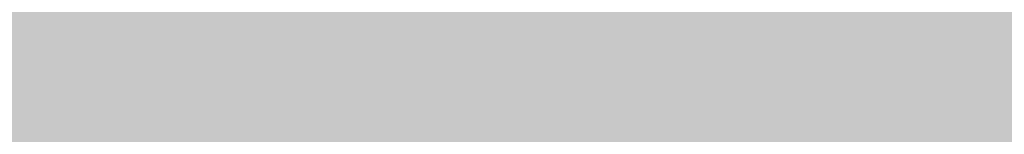
# Model space of a CAD drawing. Units: millimetres. Extents: x 0 to 2267, y 0 to 1823.
# Tile 174 of 256: x 1833.606 to 1838.83, y 1127.888 to 1128.496. Entities that reach past the tile are written whole.
import ezdxf

# ---------------------------------------------------------------- set-up
doc = ezdxf.new("R2010")
doc.units = ezdxf.units.MM
doc.header["$MEASUREMENT"] = 0
doc.layers.add('M-HATC', color=252, linetype='Continuous', lineweight=18)

msp = doc.modelspace()

# ---------------------------------------------------------------- hatches: boundary and pattern name
at = {"layer": 'M-HATC'}
h = msp.add_hatch(color=256, dxfattribs=at)
h.dxf.hatch_style = 1
h.paths.add_polyline_path([(2055.771, 1603.062), (1381.0868, 1603.062), (1381.0868, 1598.062), (2055.771, 1598.062)])
h.paths.add_polyline_path([(2055.771, 1598.062), (1381.0868, 1598.062), (1381.0868, 1593.062), (2055.771, 1593.062)])
h.paths.add_polyline_path([(2051.3074, 1536.7609), (1385.5504, 1536.7609), (1385.5504, 1526.7609), (1387.5504, 1526.7609), (1388.5366, 1525.0528), (1385.3319, 1521.2335), (1385.3319, 1521.2226), (2050.2542, 1522.7491), (2048.3212, 1525.0528), (2049.3074, 1526.7609), (2051.3074, 1526.7609)])
edge = h.paths.add_edge_path()
edge.add_arc((1847.5345, 1379.1492), 135, 222.603061, 222.890851, ccw=False)
edge.add_line((1748.1663, 1287.7656), (1683.0921, 1287.7656))
edge.add_arc((1583.7239, 1379.1492), 135, 317.109149, 317.396939, ccw=False)
edge.add_arc((1678.9686, 1290.6707), 5, 222.8909, 317.1091, ccw=False)
edge.add_arc((1774.2133, 1379.1492), 135, 222.603061, 222.890851, ccw=False)
edge.add_line((1674.8451, 1287.7656), (1609.7709, 1287.7656))
edge.add_arc((1510.4027, 1379.1492), 135, 317.109149, 317.396939, ccw=False)
edge.add_arc((1605.6474, 1290.6707), 5, 222.8909, 317.1091, ccw=False)
edge.add_arc((1700.8921, 1379.1492), 135, 222.603061, 222.890851, ccw=False)
edge.add_line((1601.5239, 1287.7656), (1536.4497, 1287.7656))
edge.add_arc((1437.0815, 1379.1492), 135, 317.109149, 317.396939, ccw=False)
edge.add_arc((1532.3262, 1290.6707), 5, 222.8909, 317.1091, ccw=False)
edge.add_arc((1627.5709, 1379.1492), 135, 222.603061, 222.890851, ccw=False)
edge.add_line((1528.2027, 1287.7656), (1505.9289, 1287.7656))
edge.add_spline(control_points=[(1505.9289, 1287.7656), (1504.2622, 1287.7656), (1504.2622, 1282.7656), (1505.9289, 1282.7656)], knot_values=[0, 0, 0, 0, 5, 5, 5, 5], degree=3, periodic=0)
edge.add_line((1505.9289, 1282.7656), (1930.9289, 1282.7656))
edge.add_spline(control_points=[(1930.9289, 1282.7656), (1932.5956, 1282.7656), (1932.5956, 1287.7656), (1930.9289, 1287.7656)], knot_values=[0, 0, 0, 0, 5, 5, 5, 5], degree=3, periodic=0)
edge.add_line((1930.9289, 1287.7656), (1903.0557, 1287.7656))
edge.add_arc((1803.6875, 1379.1492), 135, 317.109149, 317.396939, ccw=False)
edge.add_arc((1898.9322, 1290.6707), 5, 222.8909, 317.1091, ccw=False)
edge.add_arc((1994.1769, 1379.1492), 135, 222.603061, 222.890851, ccw=False)
edge.add_line((1894.8087, 1287.7656), (1829.7345, 1287.7656))
edge.add_arc((1730.3663, 1379.1492), 135, 317.109149, 317.396939, ccw=False)
edge.add_arc((1825.611, 1290.6707), 5, 222.8909, 317.1091, ccw=False)
edge.add_arc((1920.8557, 1379.1492), 135, 222.603061, 222.890851, ccw=False)
edge.add_line((1821.4875, 1287.7656), (1756.4133, 1287.7656))
edge.add_arc((1657.0451, 1379.1492), 135, 317.109149, 317.396939, ccw=False)
edge.add_arc((1752.2898, 1290.6707), 5, 222.8909, 317.1091, ccw=False)
edge = h.paths.add_edge_path()
edge.add_spline(control_points=[(1843.4289, 1227.2475), (1845.0956, 1227.2475), (1845.0956, 1232.2475), (1843.4289, 1232.2475)], knot_values=[0, 0, 0, 0, 5, 5, 5, 5], degree=3, periodic=0)
edge.add_line((1843.4289, 1232.2475), (1593.4289, 1232.2475))
edge.add_spline(control_points=[(1593.4289, 1232.2475), (1591.7622, 1232.2475), (1591.7622, 1227.2475), (1593.4289, 1227.2475)], knot_values=[0, 0, 0, 0, 5, 5, 5, 5], degree=3, periodic=0)
edge.add_line((1593.4289, 1227.2475), (1843.4289, 1227.2475))
h.paths.add_polyline_path([(1905.9289, 1127.4171), (1530.9289, 1127.4171, 0.414214), (1520.9289, 1117.4171), (1530.9289, 1117.4171), (1915.9289, 1117.4171, 0.414214)])
edge = h.paths.add_edge_path()
edge.add_arc((1397.0858, 1498.4078), 12.7299, 90.78215, 190.87871, ccw=False)
edge.add_line((1396.912, 1511.1365), (1428.0097, 1511.3488))
edge.add_line((1428.0097, 1511.3488), (1433.0097, 1511.3488))
edge.add_line((1433.0097, 1511.3488), (1434.439, 1511.3488))
edge.add_arc((1419.474, 1498.0804), 20, 41.561, 74.08211)
edge.add_line((1424.9592, 1517.3135), (1399.9351, 1517.2561))
edge.add_spline(control_points=[(1399.9307, 1517.2561), (1399.884, 1517.2131), (1399.8328, 1517.1689), (1399.7774, 1517.1236)], knot_values=[11.567499, 11.567499, 11.567499, 11.567499, 11.814249, 11.814249, 11.814249, 11.814249], degree=3, periodic=0)
edge.add_spline(control_points=[(1399.6328, 1517.0099), (1399.5831, 1516.9721), (1399.5307, 1516.9338), (1399.4759, 1516.8947)], knot_values=[11.167718, 11.167718, 11.167718, 11.167718, 11.365188, 11.365188, 11.365188, 11.365188], degree=3, periodic=0)
edge.add_spline(control_points=[(1399.3398, 1516.8001), (1399.1514, 1516.6719), (1398.9384, 1516.5377), (1398.704, 1516.3994)], knot_values=[10.376405, 10.376405, 10.376405, 10.376405, 11.00994, 11.00994, 11.00994, 11.00994], degree=3, periodic=0)
edge.add_spline(control_points=[(1398.6572, 1516.3719), (1398.5789, 1516.326), (1398.4983, 1516.2797), (1398.4155, 1516.2331)], knot_values=[10.125175, 10.125175, 10.125175, 10.125175, 10.334406, 10.334406, 10.334406, 10.334406], degree=3, periodic=0)
edge.add_spline(control_points=[(1398.2642, 1516.1487), (1398.196, 1516.1111), (1398.1263, 1516.0732), (1398.0555, 1516.0351)], knot_values=[9.832246, 9.832246, 9.832246, 9.832246, 9.999658, 9.999658, 9.999658, 9.999658], degree=3, periodic=0)
edge.add_spline(control_points=[(1397.9987, 1516.0048), (1397.7312, 1515.8621), (1397.446, 1515.7171), (1397.1466, 1515.5714)], knot_values=[9.161808, 9.161808, 9.161808, 9.161808, 9.787769, 9.787769, 9.787769, 9.787769], degree=3, periodic=0)
edge.add_spline(control_points=[(1397.1466, 1515.5714), (1396.8418, 1515.423), (1396.5222, 1515.274), (1396.1914, 1515.1262)], knot_values=[8.524455, 8.524455, 8.524455, 8.524455, 9.161808, 9.161808, 9.161808, 9.161808], degree=3, periodic=0)
edge.add_spline(control_points=[(1396.0777, 1515.0756), (1395.9854, 1515.0348), (1395.8922, 1514.994), (1395.7983, 1514.9534)], knot_values=[8.275193, 8.275193, 8.275193, 8.275193, 8.451726, 8.451726, 8.451726, 8.451726], degree=3, periodic=0)
edge.add_spline(control_points=[(1395.6018, 1514.8691), (1395.4997, 1514.8257), (1395.3968, 1514.7824), (1395.2932, 1514.7394)], knot_values=[7.962917, 7.962917, 7.962917, 7.962917, 8.152764, 8.152764, 8.152764, 8.152764], degree=3, periodic=0)
edge.add_spline(control_points=[(1395.2116, 1514.7057), (1394.8278, 1514.5475), (1394.4345, 1514.3929), (1394.0364, 1514.2442)], knot_values=[7.21254, 7.21254, 7.21254, 7.21254, 7.913148, 7.913148, 7.913148, 7.913148], degree=3, periodic=0)
edge.add_spline(control_points=[(1394.0364, 1514.2442), (1393.7076, 1514.1214), (1393.3754, 1514.0027), (1393.0427, 1513.8895)], knot_values=[6.633733, 6.633733, 6.633733, 6.633733, 7.21254, 7.21254, 7.21254, 7.21254], degree=3, periodic=0)
edge.add_spline(control_points=[(1392.8214, 1513.815), (1392.7198, 1513.7812), (1392.6181, 1513.7479), (1392.5166, 1513.7152)], knot_values=[6.328796, 6.328796, 6.328796, 6.328796, 6.505493, 6.505493, 6.505493, 6.505493], degree=3, periodic=0)
edge.add_spline(control_points=[(1392.5166, 1513.7152), (1392.3187, 1513.6515), (1392.1212, 1513.59), (1391.9244, 1513.531)], knot_values=[5.984605, 5.984605, 5.984605, 5.984605, 6.328796, 6.328796, 6.328796, 6.328796], degree=3, periodic=0)
edge.add_spline(control_points=[(1391.7915, 1513.4915), (1391.3122, 1513.3501), (1390.8384, 1513.2239), (1390.3784, 1513.1171)], knot_values=[5.066697, 5.066697, 5.066697, 5.066697, 5.907055, 5.907055, 5.907055, 5.907055], degree=3, periodic=0)
edge.add_spline(control_points=[(1390.3784, 1513.1171), (1390.1797, 1513.071), (1389.9836, 1513.0284), (1389.7907, 1512.9899)], knot_values=[4.70367, 4.70367, 4.70367, 4.70367, 5.066695, 5.066695, 5.066695, 5.066695], degree=3, periodic=0)
edge.add_spline(control_points=[(1389.422, 1512.9204), (1389.2459, 1512.8892), (1389.0729, 1512.8617), (1388.9036, 1512.8381)], knot_values=[4.130571, 4.130571, 4.130571, 4.130571, 4.469816, 4.469816, 4.469816, 4.469816], degree=3, periodic=0)
edge.add_spline(control_points=[(1388.9036, 1512.8381), (1388.591, 1512.7946), (1388.2911, 1512.7644), (1388.0071, 1512.7494)], knot_values=[3.504031, 3.504031, 3.504031, 3.504031, 4.130571, 4.130571, 4.130571, 4.130571], degree=3, periodic=0)
edge.add_spline(control_points=[(1387.9356, 1512.7459), (1387.8538, 1512.7423), (1387.7733, 1512.74), (1387.6944, 1512.739)], knot_values=[3.268866, 3.268866, 3.268866, 3.268866, 3.451164, 3.451164, 3.451164, 3.451164], degree=3, periodic=0)
edge.add_spline(control_points=[(1387.3351, 1512.7443), (1387.2076, 1512.7499), (1387.0847, 1512.7597), (1386.967, 1512.7739)], knot_values=[2.670686, 2.670686, 2.670686, 2.670686, 2.984, 2.984, 2.984, 2.984], degree=3, periodic=0)
edge.add_spline(control_points=[(1386.8327, 1512.7922), (1386.8209, 1512.7941), (1386.8092, 1512.7959), (1386.7975, 1512.7979)], knot_values=[2.516981, 2.516981, 2.516981, 2.516981, 2.549528, 2.549528, 2.549528, 2.549528], degree=3, periodic=0)
edge.add_spline(control_points=[(1386.4526, 1512.8735), (1386.4257, 1512.881), (1386.3993, 1512.889), (1386.3733, 1512.8972)], knot_values=[2.095869, 2.095869, 2.095869, 2.095869, 2.17941, 2.17941, 2.17941, 2.17941], degree=3, periodic=0)
edge.add_spline(control_points=[(1386.0691, 1513.0189), (1386.0634, 1513.0217), (1386.0577, 1513.0246), (1386.052, 1513.0275)], knot_values=[1.72453, 1.72453, 1.72453, 1.72453, 1.745933, 1.745933, 1.745933, 1.745933], degree=3, periodic=0)
edge.add_arc((1399.474, 1498.0804), 20, 131.82432, 180)
edge.add_arc((1630.3336, 1505.5484), 250.9708, 181.705176, 236.427975)
edge.add_arc((1605.3399, 1483.3044), 218.7822, 238.660829, 243.34961)
edge.add_arc((1647.0911, 1510.3592), 262.8986, 183.129836, 237.853442, ccw=False)
h.paths.add_polyline_path([(1406.5369, 1391.9644, 0.149382), (1491.5506, 1296.4418, -0.129517)], flags=17)
edge = h.paths.add_edge_path()
edge.add_arc((2037.3838, 1498.0804), 20, 0, 48.26587)
edge.add_spline(control_points=[(2050.6973, 1513.0052), (2050.6512, 1512.9847), (2050.6034, 1512.9655), (2050.5539, 1512.9477)], knot_values=[1.835652, 1.835652, 1.835652, 1.835652, 2.000781, 2.000781, 2.000781, 2.000781], degree=3, periodic=0)
edge.add_spline(control_points=[(2050.4616, 1512.9166), (2050.479, 1512.9221), (2050.4963, 1512.9277), (2050.5133, 1512.9335)], knot_values=[2.045477, 2.045477, 2.045477, 2.045477, 2.101389, 2.101389, 2.101389, 2.101389], degree=3, periodic=0)
edge.add_spline(control_points=[(2050.129, 1512.8342), (2050.1984, 1512.8473), (2050.2657, 1512.8623), (2050.3308, 1512.8792)], knot_values=[2.237629, 2.237629, 2.237629, 2.237629, 2.435841, 2.435841, 2.435841, 2.435841], degree=3, periodic=0)
edge.add_spline(control_points=[(2050.0946, 1512.8278), (2050.1061, 1512.8299), (2050.1176, 1512.832), (2050.129, 1512.8342)], knot_values=[2.435841, 2.435841, 2.435841, 2.435841, 2.468321, 2.468321, 2.468321, 2.468321], degree=3, periodic=0)
edge.add_spline(control_points=[(2049.7843, 1512.7851), (2049.8552, 1512.7922), (2049.9243, 1512.8008), (2049.9917, 1512.8109)], knot_values=[2.563852, 2.563852, 2.563852, 2.563852, 2.748541, 2.748541, 2.748541, 2.748541], degree=3, periodic=0)
edge.add_spline(control_points=[(2049.4052, 1512.7617), (2049.5364, 1512.7653), (2049.6629, 1512.773), (2049.7843, 1512.7851)], knot_values=[2.748541, 2.748541, 2.748541, 2.748541, 3.064882, 3.064882, 3.064882, 3.064882], degree=3, periodic=0)
edge.add_spline(control_points=[(2049.1698, 1512.7597), (2049.2336, 1512.7591), (2049.2965, 1512.7594), (2049.3584, 1512.7606)], knot_values=[3.102309, 3.102309, 3.102309, 3.102309, 3.2503, 3.2503, 3.2503, 3.2503], degree=3, periodic=0)
edge.add_spline(control_points=[(2048.8573, 1512.7691), (2048.9638, 1512.7638), (2049.068, 1512.7606), (2049.1698, 1512.7597)], knot_values=[3.2503, 3.2503, 3.2503, 3.2503, 3.486069, 3.486069, 3.486069, 3.486069], degree=3, periodic=0)
edge.add_spline(control_points=[(2048.6924, 1512.7789), (2048.3729, 1512.8009), (2048.0345, 1512.8411), (2047.6817, 1512.897)], knot_values=[3.606429, 3.606429, 3.606429, 3.606429, 4.2989, 4.2989, 4.2989, 4.2989], degree=3, periodic=0)
edge.add_spline(control_points=[(2047.6817, 1512.897), (2047.5458, 1512.9185), (2047.4077, 1512.9424), (2047.2678, 1512.9685)], knot_values=[4.2989, 4.2989, 4.2989, 4.2989, 4.565769, 4.565769, 4.565769, 4.565769], degree=3, periodic=0)
edge.add_spline(control_points=[(2047.2678, 1512.9685), (2047.1449, 1512.9914), (2047.0207, 1513.016), (2046.8951, 1513.0422)], knot_values=[4.565769, 4.565769, 4.565769, 4.565769, 4.799971, 4.799971, 4.799971, 4.799971], degree=3, periodic=0)
edge.add_spline(control_points=[(2046.8951, 1513.0422), (2046.5286, 1513.1188), (2046.1513, 1513.209), (2045.7676, 1513.3107)], knot_values=[4.799971, 4.799971, 4.799971, 4.799971, 5.483718, 5.483718, 5.483718, 5.483718], degree=3, periodic=0)
edge.add_spline(control_points=[(2045.7676, 1513.3107), (2045.3724, 1513.4154), (2044.9704, 1513.5322), (2044.5662, 1513.6588)], knot_values=[5.483718, 5.483718, 5.483718, 5.483718, 6.187866, 6.187866, 6.187866, 6.187866], degree=3, periodic=0)
edge.add_spline(control_points=[(2044.5662, 1513.6588), (2044.4149, 1513.7061), (2044.2633, 1513.7549), (2044.1116, 1513.8048)], knot_values=[6.187866, 6.187866, 6.187866, 6.187866, 6.451551, 6.451551, 6.451551, 6.451551], degree=3, periodic=0)
edge.add_spline(control_points=[(2044.1116, 1513.8048), (2043.9967, 1513.8427), (2043.8817, 1513.8813), (2043.7668, 1513.9205)], knot_values=[6.451551, 6.451551, 6.451551, 6.451551, 6.651434, 6.651434, 6.651434, 6.651434], degree=3, periodic=0)
edge.add_spline(control_points=[(2043.7668, 1513.9205), (2043.3716, 1514.0554), (2042.9774, 1514.1979), (2042.5886, 1514.3458)], knot_values=[6.651434, 6.651434, 6.651434, 6.651434, 7.338879, 7.338879, 7.338879, 7.338879], degree=3, periodic=0)
edge.add_spline(control_points=[(2042.5886, 1514.3458), (2042.1643, 1514.5071), (2041.7465, 1514.6749), (2041.3409, 1514.846)], knot_values=[7.338879, 7.338879, 7.338879, 7.338879, 8.089209, 8.089209, 8.089209, 8.089209], degree=3, periodic=0)
edge.add_spline(control_points=[(2041.3409, 1514.846), (2041.1028, 1514.9465), (2040.869, 1515.0481), (2040.6405, 1515.1502)], knot_values=[8.089209, 8.089209, 8.089209, 8.089209, 8.529587, 8.529587, 8.529587, 8.529587], degree=3, periodic=0)
edge.add_spline(control_points=[(2040.51, 1515.2089), (2040.0824, 1515.4022), (2039.6747, 1515.5971), (2039.295, 1515.7894)], knot_values=[8.613818, 8.613818, 8.613818, 8.613818, 9.44571, 9.44571, 9.44571, 9.44571], degree=3, periodic=0)
edge.add_spline(control_points=[(2039.295, 1515.7894), (2039.0618, 1515.9075), (2038.8391, 1516.0246), (2038.6288, 1516.1398)], knot_values=[9.44571, 9.44571, 9.44571, 9.44571, 9.956404, 9.956404, 9.956404, 9.956404], degree=3, periodic=0)
edge.add_spline(control_points=[(2038.6288, 1516.1398), (2038.5187, 1516.2001), (2038.4121, 1516.2598), (2038.309, 1516.3189)], knot_values=[9.956404, 9.956404, 9.956404, 9.956404, 10.223542, 10.223542, 10.223542, 10.223542], degree=3, periodic=0)
edge.add_spline(control_points=[(2038.309, 1516.3189), (2038.2138, 1516.3735), (2038.1216, 1516.4276), (2038.0328, 1516.481)], knot_values=[10.223542, 10.223542, 10.223542, 10.223542, 10.47051, 10.47051, 10.47051, 10.47051], degree=3, periodic=0)
edge.add_spline(control_points=[(2038.0328, 1516.481), (2037.7855, 1516.6296), (2037.5639, 1516.773), (2037.3722, 1516.909)], knot_values=[10.47051, 10.47051, 10.47051, 10.47051, 11.15767, 11.15767, 11.15767, 11.15767], degree=3, periodic=0)
edge.add_spline(control_points=[(2037.3722, 1516.909), (2037.2789, 1516.9752), (2037.1927, 1517.0396), (2037.1142, 1517.102)], knot_values=[11.15767, 11.15767, 11.15767, 11.15767, 11.49227, 11.49227, 11.49227, 11.49227], degree=3, periodic=0)
edge.add_spline(control_points=[(2036.8564, 1517.3259), (2036.9148, 1517.2692), (2036.9814, 1517.2103), (2037.0557, 1517.1492)], knot_values=[11.577341, 11.577341, 11.577341, 11.577341, 11.91035, 11.91035, 11.91035, 11.91035], degree=3, periodic=0)
edge.add_spline(control_points=[(2036.8074, 1517.3748), (2036.823, 1517.3587), (2036.8393, 1517.3424), (2036.8564, 1517.3259)], knot_values=[11.91035, 11.91035, 11.91035, 11.91035, 12.007402, 12.007402, 12.007402, 12.007402], degree=3, periodic=0)
edge.add_spline(control_points=[(2036.7017, 1517.494), (2036.7104, 1517.483), (2036.7196, 1517.4719), (2036.7291, 1517.4606)], knot_values=[12.184155, 12.184155, 12.184155, 12.184155, 12.255409, 12.255409, 12.255409, 12.255409], degree=3, periodic=0)
edge.add_spline(control_points=[(2036.6159, 1517.6205), (2036.62, 1517.613), (2036.6243, 1517.6055), (2036.6289, 1517.5979)], knot_values=[12.487913, 12.487913, 12.487913, 12.487913, 12.541035, 12.541035, 12.541035, 12.541035], degree=3, periodic=0)
edge.add_spline(control_points=[(2036.5635, 1517.786), (2036.5637, 1517.7794), (2036.5642, 1517.7726), (2036.565, 1517.7658)], knot_values=[12.911761, 12.911761, 12.911761, 12.911761, 12.968286, 12.968286, 12.968286, 12.968286], degree=3, periodic=0)
edge.add_spline(control_points=[(2036.6166, 1517.9304), (2036.6125, 1517.9259), (2036.6086, 1517.9212), (2036.6049, 1517.9165)], knot_values=[13.382527, 13.382527, 13.382527, 13.382527, 13.433791, 13.433791, 13.433791, 13.433791], degree=3, periodic=0)
edge.add_spline(control_points=[(2036.749, 1518.017), (2036.7361, 1518.0116), (2036.7239, 1518.006), (2036.7124, 1518.0002)], knot_values=[13.726299, 13.726299, 13.726299, 13.726299, 13.809928, 13.809928, 13.809928, 13.809928], degree=3, periodic=0)
edge.add_spline(control_points=[(2036.8604, 1518.0528), (2036.8386, 1518.0474), (2036.8181, 1518.0416), (2036.7988, 1518.0353)], knot_values=[13.910887, 13.910887, 13.910887, 13.910887, 14.02153, 14.02153, 14.02153, 14.02153], degree=3, periodic=0)
edge.add_line((2036.9639, 1518.0804), (2032.3838, 1518.0804))
edge.add_line((2032.3838, 1518.0804), (2027.3838, 1518.0804))
edge.add_line((2027.3838, 1518.0804), (2022.3838, 1518.0804))
edge.add_line((2022.3838, 1518.0804), (2017.3838, 1518.0804))
edge.add_arc((2017.3838, 1498.0804), 20, 90, 138.439)
edge.add_line((2002.4188, 1511.3488), (2003.8481, 1511.3488))
edge.add_line((2003.8481, 1511.3488), (2008.8481, 1511.3488))
edge.add_line((2008.8481, 1511.3488), (2039.772, 1511.1377))
edge.add_arc((2039.772, 1498.4078), 12.7299, -10.87871, 90, ccw=False)
edge.add_arc((1789.7668, 1510.3592), 262.8986, 302.146558, 356.870164, ccw=False)
edge.add_arc((1831.5179, 1483.3044), 218.7822, 296.65039, 301.339171)
edge.add_arc((1806.5242, 1505.5484), 250.9708, 303.572025, 358.294824)
h.paths.add_polyline_path([(2030.321, 1391.9644, -0.129517), (1945.3072, 1296.4418, 0.149382)], flags=17)
edge = h.paths.add_edge_path()
edge.add_spline(control_points=[(2037.2464, 1518.0821), (2037.2898, 1518.081), (2037.3355, 1518.0804), (2037.3838, 1518.0804)], knot_values=[0.000012, 0.000012, 0.000012, 0.000012, 0.144754, 0.144754, 0.144754, 0.144754], degree=3, periodic=0)
edge.add_line((2037.3357, 1518.0804), (2037.0096, 1518.0804))
edge.add_spline(control_points=[(2037.0096, 1518.0804), (2036.9822, 1518.0768), (2036.956, 1518.0727), (2036.9312, 1518.0681)], knot_values=[14.13465, 14.13465, 14.13465, 14.13465, 14.247197, 14.247197, 14.247197, 14.247197], degree=3, periodic=0)
edge.add_spline(control_points=[(2036.9312, 1518.0681), (2036.9276, 1518.0674), (2036.9241, 1518.0667), (2036.9205, 1518.0661)], knot_values=[14.118315, 14.118315, 14.118315, 14.118315, 14.13465, 14.13465, 14.13465, 14.13465], degree=3, periodic=0)
edge.add_spline(control_points=[(2036.9205, 1518.0661), (2036.9118, 1518.0644), (2036.9032, 1518.0626), (2036.8948, 1518.0608)], knot_values=[14.078086, 14.078086, 14.078086, 14.078086, 14.118315, 14.118315, 14.118315, 14.118315], degree=3, periodic=0)
edge.add_spline(control_points=[(2036.8948, 1518.0608), (2036.883, 1518.0583), (2036.8716, 1518.0556), (2036.8604, 1518.0528)], knot_values=[14.02153, 14.02153, 14.02153, 14.02153, 14.078086, 14.078086, 14.078086, 14.078086], degree=3, periodic=0)
edge.add_spline(control_points=[(2036.8604, 1518.0528), (2036.8386, 1518.0474), (2036.8181, 1518.0416), (2036.7988, 1518.0353)], knot_values=[13.910887, 13.910887, 13.910887, 13.910887, 14.02153, 14.02153, 14.02153, 14.02153], degree=3, periodic=0)
edge.add_spline(control_points=[(2036.7988, 1518.0353), (2036.7981, 1518.035), (2036.7974, 1518.0348), (2036.7967, 1518.0346)], knot_values=[13.906906, 13.906906, 13.906906, 13.906906, 13.910887, 13.910887, 13.910887, 13.910887], degree=3, periodic=0)
edge.add_spline(control_points=[(2036.7967, 1518.0346), (2036.7882, 1518.0318), (2036.7799, 1518.0289), (2036.7719, 1518.0259)], knot_values=[13.857826, 13.857826, 13.857826, 13.857826, 13.906906, 13.906906, 13.906906, 13.906906], degree=3, periodic=0)
edge.add_spline(control_points=[(2036.7719, 1518.0259), (2036.764, 1518.023), (2036.7564, 1518.02), (2036.749, 1518.017)], knot_values=[13.809928, 13.809928, 13.809928, 13.809928, 13.857826, 13.857826, 13.857826, 13.857826], degree=3, periodic=0)
edge.add_spline(control_points=[(2036.749, 1518.017), (2036.7361, 1518.0116), (2036.7239, 1518.006), (2036.7124, 1518.0002)], knot_values=[13.726299, 13.726299, 13.726299, 13.726299, 13.809928, 13.809928, 13.809928, 13.809928], degree=3, periodic=0)
edge.add_spline(control_points=[(2036.7124, 1518.0002), (2036.7121, 1518), (2036.7118, 1517.9999), (2036.7115, 1517.9997)], knot_values=[13.723993, 13.723993, 13.723993, 13.723993, 13.726299, 13.726299, 13.726299, 13.726299], degree=3, periodic=0)
edge.add_spline(control_points=[(2036.7115, 1517.9997), (2036.7063, 1517.9971), (2036.7013, 1517.9944), (2036.6965, 1517.9917)], knot_values=[13.686536, 13.686536, 13.686536, 13.686536, 13.723993, 13.723993, 13.723993, 13.723993], degree=3, periodic=0)
edge.add_spline(control_points=[(2036.6965, 1517.9917), (2036.6919, 1517.9891), (2036.6874, 1517.9865), (2036.6831, 1517.9839)], knot_values=[13.651251, 13.651251, 13.651251, 13.651251, 13.686536, 13.686536, 13.686536, 13.686536], degree=3, periodic=0)
edge.add_spline(control_points=[(2036.6831, 1517.9839), (2036.6764, 1517.9798), (2036.67, 1517.9757), (2036.6639, 1517.9714)], knot_values=[13.596804, 13.596804, 13.596804, 13.596804, 13.651251, 13.651251, 13.651251, 13.651251], degree=3, periodic=0)
edge.add_spline(control_points=[(2036.6639, 1517.9714), (2036.6636, 1517.9712), (2036.6633, 1517.9709), (2036.6629, 1517.9707)], knot_values=[13.593956, 13.593956, 13.593956, 13.593956, 13.596804, 13.596804, 13.596804, 13.596804], degree=3, periodic=0)
edge.add_spline(control_points=[(2036.6629, 1517.9707), (2036.6603, 1517.9689), (2036.6577, 1517.967), (2036.6552, 1517.9651)], knot_values=[13.570322, 13.570322, 13.570322, 13.570322, 13.593956, 13.593956, 13.593956, 13.593956], degree=3, periodic=0)
edge.add_spline(control_points=[(2036.6552, 1517.9651), (2036.6525, 1517.9631), (2036.6499, 1517.9611), (2036.6474, 1517.9591)], knot_values=[13.545477, 13.545477, 13.545477, 13.545477, 13.570322, 13.570322, 13.570322, 13.570322], degree=3, periodic=0)
edge.add_spline(control_points=[(2036.6474, 1517.9591), (2036.6472, 1517.9589), (2036.6471, 1517.9588), (2036.6469, 1517.9587)], knot_values=[13.543931, 13.543931, 13.543931, 13.543931, 13.545477, 13.545477, 13.545477, 13.545477], degree=3, periodic=0)
edge.add_spline(control_points=[(2036.6469, 1517.9587), (2036.6412, 1517.9541), (2036.6358, 1517.9494), (2036.6307, 1517.9447)], knot_values=[13.488237, 13.488237, 13.488237, 13.488237, 13.543931, 13.543931, 13.543931, 13.543931], degree=3, periodic=0)
edge.add_spline(control_points=[(2036.6307, 1517.9447), (2036.6282, 1517.9423), (2036.6257, 1517.9399), (2036.6233, 1517.9374)], knot_values=[13.460307, 13.460307, 13.460307, 13.460307, 13.488237, 13.488237, 13.488237, 13.488237], degree=3, periodic=0)
edge.add_spline(control_points=[(2036.6233, 1517.9374), (2036.6215, 1517.9356), (2036.6198, 1517.9338), (2036.6181, 1517.932)], knot_values=[13.439712, 13.439712, 13.439712, 13.439712, 13.460307, 13.460307, 13.460307, 13.460307], degree=3, periodic=0)
edge.add_spline(control_points=[(2036.6181, 1517.932), (2036.6176, 1517.9315), (2036.6171, 1517.9309), (2036.6166, 1517.9304)], knot_values=[13.433791, 13.433791, 13.433791, 13.433791, 13.439712, 13.439712, 13.439712, 13.439712], degree=3, periodic=0)
edge.add_spline(control_points=[(2036.6166, 1517.9304), (2036.6125, 1517.9259), (2036.6086, 1517.9212), (2036.6049, 1517.9165)], knot_values=[13.382527, 13.382527, 13.382527, 13.382527, 13.433791, 13.433791, 13.433791, 13.433791], degree=3, periodic=0)
edge.add_spline(control_points=[(2036.6049, 1517.9165), (2036.6026, 1517.9135), (2036.6004, 1517.9104), (2036.5982, 1517.9074)], knot_values=[13.350017, 13.350017, 13.350017, 13.350017, 13.382527, 13.382527, 13.382527, 13.382527], degree=3, periodic=0)
edge.add_spline(control_points=[(2036.5982, 1517.9074), (2036.5972, 1517.9059), (2036.5962, 1517.9043), (2036.5952, 1517.9028)], knot_values=[13.333922, 13.333922, 13.333922, 13.333922, 13.350017, 13.350017, 13.350017, 13.350017], degree=3, periodic=0)
edge.add_spline(control_points=[(2036.5952, 1517.9028), (2036.5945, 1517.9018), (2036.5939, 1517.9009), (2036.5933, 1517.8999)], knot_values=[13.323828, 13.323828, 13.323828, 13.323828, 13.333922, 13.333922, 13.333922, 13.333922], degree=3, periodic=0)
edge.add_spline(control_points=[(2036.5933, 1517.8999), (2036.5905, 1517.8955), (2036.5879, 1517.8909), (2036.5855, 1517.8864)], knot_values=[13.277545, 13.277545, 13.277545, 13.277545, 13.323828, 13.323828, 13.323828, 13.323828], degree=3, periodic=0)
edge.add_spline(control_points=[(2036.5855, 1517.8864), (2036.5836, 1517.8827), (2036.5817, 1517.8789), (2036.5801, 1517.8751)], knot_values=[13.240119, 13.240119, 13.240119, 13.240119, 13.277545, 13.277545, 13.277545, 13.277545], degree=3, periodic=0)
edge.add_spline(control_points=[(2036.5801, 1517.8751), (2036.5795, 1517.8739), (2036.579, 1517.8727), (2036.5785, 1517.8715)], knot_values=[13.228211, 13.228211, 13.228211, 13.228211, 13.240119, 13.240119, 13.240119, 13.240119], degree=3, periodic=0)
edge.add_spline(control_points=[(2036.5785, 1517.8715), (2036.578, 1517.8702), (2036.5774, 1517.869), (2036.5769, 1517.8677)], knot_values=[13.215717, 13.215717, 13.215717, 13.215717, 13.228211, 13.228211, 13.228211, 13.228211], degree=3, periodic=0)
edge.add_spline(control_points=[(2036.5769, 1517.8677), (2036.5755, 1517.864), (2036.5741, 1517.8603), (2036.5729, 1517.8565)], knot_values=[13.179847, 13.179847, 13.179847, 13.179847, 13.215717, 13.215717, 13.215717, 13.215717], degree=3, periodic=0)
edge.add_spline(control_points=[(2036.5729, 1517.8565), (2036.5713, 1517.8515), (2036.5699, 1517.8464), (2036.5687, 1517.8413)], knot_values=[13.132017, 13.132017, 13.132017, 13.132017, 13.179847, 13.179847, 13.179847, 13.179847], degree=3, periodic=0)
edge.add_spline(control_points=[(2036.5687, 1517.8413), (2036.5684, 1517.8402), (2036.5682, 1517.8392), (2036.568, 1517.8382)], knot_values=[13.122482, 13.122482, 13.122482, 13.122482, 13.132017, 13.132017, 13.132017, 13.132017], degree=3, periodic=0)
edge.add_spline(control_points=[(2036.568, 1517.8382), (2036.5676, 1517.8363), (2036.5672, 1517.8345), (2036.5669, 1517.8327)], knot_values=[13.105592, 13.105592, 13.105592, 13.105592, 13.122482, 13.122482, 13.122482, 13.122482], degree=3, periodic=0)
edge.add_spline(control_points=[(2036.5669, 1517.8327), (2036.5662, 1517.8292), (2036.5657, 1517.8257), (2036.5652, 1517.8222)], knot_values=[13.074063, 13.074063, 13.074063, 13.074063, 13.105592, 13.105592, 13.105592, 13.105592], degree=3, periodic=0)
edge.add_spline(control_points=[(2036.5652, 1517.8222), (2036.5652, 1517.8222), (2036.5652, 1517.8222), (2036.5652, 1517.8222)], knot_values=[13.074043, 13.074043, 13.074043, 13.074043, 13.074063, 13.074063, 13.074063, 13.074063], degree=3, periodic=0)
edge.add_spline(control_points=[(2036.5652, 1517.8222), (2036.5644, 1517.8164), (2036.5639, 1517.8106), (2036.5636, 1517.8046)], knot_values=[13.021884, 13.021884, 13.021884, 13.021884, 13.074043, 13.074043, 13.074043, 13.074043], degree=3, periodic=0)
edge.add_spline(control_points=[(2036.5636, 1517.8046), (2036.5636, 1517.804), (2036.5636, 1517.8034), (2036.5635, 1517.8028)], knot_values=[13.01674, 13.01674, 13.01674, 13.01674, 13.021884, 13.021884, 13.021884, 13.021884], degree=3, periodic=0)
edge.add_spline(control_points=[(2036.5635, 1517.8028), (2036.5634, 1517.8005), (2036.5634, 1517.7982), (2036.5634, 1517.7958)], knot_values=[12.996438, 12.996438, 12.996438, 12.996438, 13.01674, 13.01674, 13.01674, 13.01674], degree=3, periodic=0)
edge.add_spline(control_points=[(2036.5634, 1517.7958), (2036.5633, 1517.7926), (2036.5634, 1517.7893), (2036.5635, 1517.786)], knot_values=[12.968286, 12.968286, 12.968286, 12.968286, 12.996438, 12.996438, 12.996438, 12.996438], degree=3, periodic=0)
edge.add_spline(control_points=[(2036.5635, 1517.786), (2036.5637, 1517.7794), (2036.5642, 1517.7726), (2036.565, 1517.7658)], knot_values=[12.911761, 12.911761, 12.911761, 12.911761, 12.968286, 12.968286, 12.968286, 12.968286], degree=3, periodic=0)
edge.add_spline(control_points=[(2036.565, 1517.7658), (2036.565, 1517.7657), (2036.565, 1517.7656), (2036.565, 1517.7656)], knot_values=[12.911017, 12.911017, 12.911017, 12.911017, 12.911761, 12.911761, 12.911761, 12.911761], degree=3, periodic=0)
edge.add_spline(control_points=[(2036.565, 1517.7656), (2036.5654, 1517.7625), (2036.5658, 1517.7593), (2036.5663, 1517.7562)], knot_values=[12.88528, 12.88528, 12.88528, 12.88528, 12.911017, 12.911017, 12.911017, 12.911017], degree=3, periodic=0)
edge.add_spline(control_points=[(2036.5663, 1517.7562), (2036.5667, 1517.7534), (2036.5672, 1517.7506), (2036.5677, 1517.7478)], knot_values=[12.862519, 12.862519, 12.862519, 12.862519, 12.88528, 12.88528, 12.88528, 12.88528], degree=3, periodic=0)
edge.add_spline(control_points=[(2036.5677, 1517.7478), (2036.5678, 1517.7474), (2036.5679, 1517.7469), (2036.568, 1517.7465)], knot_values=[12.858885, 12.858885, 12.858885, 12.858885, 12.862519, 12.862519, 12.862519, 12.862519], degree=3, periodic=0)
edge.add_spline(control_points=[(2036.568, 1517.7465), (2036.5692, 1517.7399), (2036.5707, 1517.7332), (2036.5724, 1517.7264)], knot_values=[12.8053, 12.8053, 12.8053, 12.8053, 12.858885, 12.858885, 12.858885, 12.858885], degree=3, periodic=0)
edge.add_spline(control_points=[(2036.5724, 1517.7264), (2036.5734, 1517.7226), (2036.5745, 1517.7187), (2036.5756, 1517.7149)], knot_values=[12.775176, 12.775176, 12.775176, 12.775176, 12.8053, 12.8053, 12.8053, 12.8053], degree=3, periodic=0)
edge.add_spline(control_points=[(2036.5756, 1517.7149), (2036.5763, 1517.7125), (2036.577, 1517.7102), (2036.5778, 1517.7078)], knot_values=[12.756759, 12.756759, 12.756759, 12.756759, 12.775176, 12.775176, 12.775176, 12.775176], degree=3, periodic=0)
edge.add_spline(control_points=[(2036.5778, 1517.7078), (2036.5781, 1517.7067), (2036.5784, 1517.7057), (2036.5787, 1517.7047)], knot_values=[12.748742, 12.748742, 12.748742, 12.748742, 12.756759, 12.756759, 12.756759, 12.756759], degree=3, periodic=0)
edge.add_spline(control_points=[(2036.5787, 1517.7047), (2036.5808, 1517.6983), (2036.5831, 1517.6919), (2036.5856, 1517.6854)], knot_values=[12.69959, 12.69959, 12.69959, 12.69959, 12.748742, 12.748742, 12.748742, 12.748742], degree=3, periodic=0)
edge.add_spline(control_points=[(2036.5856, 1517.6854), (2036.5876, 1517.68), (2036.5898, 1517.6746), (2036.5921, 1517.6692)], knot_values=[12.659038, 12.659038, 12.659038, 12.659038, 12.69959, 12.69959, 12.69959, 12.69959], degree=3, periodic=0)
edge.add_spline(control_points=[(2036.5921, 1517.6692), (2036.594, 1517.6648), (2036.5959, 1517.6605), (2036.5979, 1517.6561)], knot_values=[12.626806, 12.626806, 12.626806, 12.626806, 12.659038, 12.659038, 12.659038, 12.659038], degree=3, periodic=0)
edge.add_spline(control_points=[(2036.5979, 1517.6561), (2036.5984, 1517.6551), (2036.5989, 1517.6541), (2036.5993, 1517.6531)], knot_values=[12.619394, 12.619394, 12.619394, 12.619394, 12.626806, 12.626806, 12.626806, 12.626806], degree=3, periodic=0)
edge.add_spline(control_points=[(2036.5993, 1517.6531), (2036.6043, 1517.6424), (2036.6099, 1517.6315), (2036.6159, 1517.6205)], knot_values=[12.541039, 12.541039, 12.541039, 12.541039, 12.619394, 12.619394, 12.619394, 12.619394], degree=3, periodic=0)
edge.add_spline(control_points=[(2036.6159, 1517.6205), (2036.6159, 1517.6205), (2036.6159, 1517.6205), (2036.6159, 1517.6205)], knot_values=[12.541035, 12.541035, 12.541035, 12.541035, 12.541039, 12.541039, 12.541039, 12.541039], degree=3, periodic=0)
edge.add_spline(control_points=[(2036.6159, 1517.6205), (2036.62, 1517.613), (2036.6243, 1517.6055), (2036.6289, 1517.5979)], knot_values=[12.487913, 12.487913, 12.487913, 12.487913, 12.541035, 12.541035, 12.541035, 12.541035], degree=3, periodic=0)
edge.add_spline(control_points=[(2036.6289, 1517.5979), (2036.6326, 1517.5916), (2036.6365, 1517.5853), (2036.6406, 1517.5789)], knot_values=[12.443982, 12.443982, 12.443982, 12.443982, 12.487913, 12.487913, 12.487913, 12.487913], degree=3, periodic=0)
edge.add_spline(control_points=[(2036.6406, 1517.5789), (2036.6414, 1517.5776), (2036.6423, 1517.5763), (2036.6431, 1517.5749)], knot_values=[12.434996, 12.434996, 12.434996, 12.434996, 12.443982, 12.443982, 12.443982, 12.443982], degree=3, periodic=0)
edge.add_spline(control_points=[(2036.6431, 1517.5749), (2036.6531, 1517.5596), (2036.6639, 1517.5439), (2036.6756, 1517.528)], knot_values=[12.329647, 12.329647, 12.329647, 12.329647, 12.434996, 12.434996, 12.434996, 12.434996], degree=3, periodic=0)
edge.add_spline(control_points=[(2036.6756, 1517.528), (2036.6839, 1517.5168), (2036.6925, 1517.5055), (2036.7017, 1517.494)], knot_values=[12.255409, 12.255409, 12.255409, 12.255409, 12.329647, 12.329647, 12.329647, 12.329647], degree=3, periodic=0)
edge.add_spline(control_points=[(2036.7017, 1517.494), (2036.7104, 1517.483), (2036.7196, 1517.4719), (2036.7291, 1517.4606)], knot_values=[12.184155, 12.184155, 12.184155, 12.184155, 12.255409, 12.255409, 12.255409, 12.255409], degree=3, periodic=0)
edge.add_spline(control_points=[(2036.7291, 1517.4606), (2036.7436, 1517.4435), (2036.759, 1517.4262), (2036.7753, 1517.4085)], knot_values=[12.075961, 12.075961, 12.075961, 12.075961, 12.184155, 12.184155, 12.184155, 12.184155], degree=3, periodic=0)
edge.add_spline(control_points=[(2036.7753, 1517.4085), (2036.7763, 1517.4075), (2036.7773, 1517.4064), (2036.7783, 1517.4054)], knot_values=[12.069502, 12.069502, 12.069502, 12.069502, 12.075961, 12.075961, 12.075961, 12.075961], degree=3, periodic=0)
edge.add_spline(control_points=[(2036.7783, 1517.4054), (2036.7877, 1517.3953), (2036.7974, 1517.385), (2036.8074, 1517.3748)], knot_values=[12.007402, 12.007402, 12.007402, 12.007402, 12.069502, 12.069502, 12.069502, 12.069502], degree=3, periodic=0)
edge.add_spline(control_points=[(2036.8074, 1517.3748), (2036.823, 1517.3587), (2036.8393, 1517.3424), (2036.8564, 1517.3259)], knot_values=[11.91035, 11.91035, 11.91035, 11.91035, 12.007402, 12.007402, 12.007402, 12.007402], degree=3, periodic=0)
edge.add_spline(control_points=[(2036.8564, 1517.3259), (2036.9148, 1517.2692), (2036.9814, 1517.2103), (2037.0557, 1517.1492)], knot_values=[11.577341, 11.577341, 11.577341, 11.577341, 11.91035, 11.91035, 11.91035, 11.91035], degree=3, periodic=0)
edge.add_spline(control_points=[(2037.0557, 1517.1492), (2037.0747, 1517.1336), (2037.0942, 1517.1179), (2037.1142, 1517.102)], knot_values=[11.49227, 11.49227, 11.49227, 11.49227, 11.577341, 11.577341, 11.577341, 11.577341], degree=3, periodic=0)
edge.add_spline(control_points=[(2037.1142, 1517.102), (2037.1927, 1517.0396), (2037.2789, 1516.9752), (2037.3722, 1516.909)], knot_values=[11.15767, 11.15767, 11.15767, 11.15767, 11.49227, 11.49227, 11.49227, 11.49227], degree=3, periodic=0)
edge.add_spline(control_points=[(2037.3722, 1516.909), (2037.5639, 1516.773), (2037.7855, 1516.6296), (2038.0328, 1516.481)], knot_values=[10.47051, 10.47051, 10.47051, 10.47051, 11.15767, 11.15767, 11.15767, 11.15767], degree=3, periodic=0)
edge.add_spline(control_points=[(2038.0328, 1516.481), (2038.1216, 1516.4276), (2038.2138, 1516.3735), (2038.309, 1516.3189)], knot_values=[10.223542, 10.223542, 10.223542, 10.223542, 10.47051, 10.47051, 10.47051, 10.47051], degree=3, periodic=0)
edge.add_spline(control_points=[(2038.309, 1516.3189), (2038.4121, 1516.2598), (2038.5187, 1516.2001), (2038.6288, 1516.1398)], knot_values=[9.956404, 9.956404, 9.956404, 9.956404, 10.223542, 10.223542, 10.223542, 10.223542], degree=3, periodic=0)
edge.add_spline(control_points=[(2038.6288, 1516.1398), (2038.8391, 1516.0246), (2039.0618, 1515.9075), (2039.295, 1515.7894)], knot_values=[9.44571, 9.44571, 9.44571, 9.44571, 9.956404, 9.956404, 9.956404, 9.956404], degree=3, periodic=0)
edge.add_spline(control_points=[(2039.295, 1515.7894), (2039.6747, 1515.5971), (2040.0824, 1515.4022), (2040.51, 1515.2089)], knot_values=[8.613818, 8.613818, 8.613818, 8.613818, 9.44571, 9.44571, 9.44571, 9.44571], degree=3, periodic=0)
edge.add_spline(control_points=[(2040.51, 1515.2089), (2040.5533, 1515.1893), (2040.5968, 1515.1697), (2040.6405, 1515.1502)], knot_values=[8.529587, 8.529587, 8.529587, 8.529587, 8.613818, 8.613818, 8.613818, 8.613818], degree=3, periodic=0)
edge.add_spline(control_points=[(2040.6405, 1515.1502), (2040.869, 1515.0481), (2041.1028, 1514.9465), (2041.3409, 1514.846)], knot_values=[8.089209, 8.089209, 8.089209, 8.089209, 8.529587, 8.529587, 8.529587, 8.529587], degree=3, periodic=0)
edge.add_spline(control_points=[(2041.3409, 1514.846), (2041.7465, 1514.6749), (2042.1643, 1514.5071), (2042.5886, 1514.3458)], knot_values=[7.338879, 7.338879, 7.338879, 7.338879, 8.089209, 8.089209, 8.089209, 8.089209], degree=3, periodic=0)
edge.add_spline(control_points=[(2042.5886, 1514.3458), (2042.9774, 1514.1979), (2043.3716, 1514.0554), (2043.7668, 1513.9205)], knot_values=[6.651434, 6.651434, 6.651434, 6.651434, 7.338879, 7.338879, 7.338879, 7.338879], degree=3, periodic=0)
edge.add_spline(control_points=[(2043.7668, 1513.9205), (2043.8817, 1513.8813), (2043.9967, 1513.8427), (2044.1116, 1513.8048)], knot_values=[6.451551, 6.451551, 6.451551, 6.451551, 6.651434, 6.651434, 6.651434, 6.651434], degree=3, periodic=0)
edge.add_spline(control_points=[(2044.1116, 1513.8048), (2044.2633, 1513.7549), (2044.4149, 1513.7061), (2044.5662, 1513.6588)], knot_values=[6.187866, 6.187866, 6.187866, 6.187866, 6.451551, 6.451551, 6.451551, 6.451551], degree=3, periodic=0)
edge.add_spline(control_points=[(2044.5662, 1513.6588), (2044.9704, 1513.5322), (2045.3724, 1513.4154), (2045.7676, 1513.3107)], knot_values=[5.483718, 5.483718, 5.483718, 5.483718, 6.187866, 6.187866, 6.187866, 6.187866], degree=3, periodic=0)
edge.add_spline(control_points=[(2045.7676, 1513.3107), (2046.1513, 1513.209), (2046.5286, 1513.1188), (2046.8951, 1513.0422)], knot_values=[4.799971, 4.799971, 4.799971, 4.799971, 5.483718, 5.483718, 5.483718, 5.483718], degree=3, periodic=0)
edge.add_spline(control_points=[(2046.8951, 1513.0422), (2047.0207, 1513.016), (2047.1449, 1512.9914), (2047.2678, 1512.9685)], knot_values=[4.565769, 4.565769, 4.565769, 4.565769, 4.799971, 4.799971, 4.799971, 4.799971], degree=3, periodic=0)
edge.add_spline(control_points=[(2047.2678, 1512.9685), (2047.4077, 1512.9424), (2047.5458, 1512.9185), (2047.6817, 1512.897)], knot_values=[4.2989, 4.2989, 4.2989, 4.2989, 4.565769, 4.565769, 4.565769, 4.565769], degree=3, periodic=0)
edge.add_spline(control_points=[(2047.6817, 1512.897), (2048.0345, 1512.8411), (2048.3729, 1512.8009), (2048.6924, 1512.7789)], knot_values=[3.606429, 3.606429, 3.606429, 3.606429, 4.2989, 4.2989, 4.2989, 4.2989], degree=3, periodic=0)
edge.add_spline(control_points=[(2048.6924, 1512.7789), (2048.7479, 1512.7751), (2048.8029, 1512.7718), (2048.8573, 1512.7691)], knot_values=[3.486069, 3.486069, 3.486069, 3.486069, 3.606429, 3.606429, 3.606429, 3.606429], degree=3, periodic=0)
edge.add_spline(control_points=[(2048.8573, 1512.7691), (2048.9638, 1512.7638), (2049.068, 1512.7606), (2049.1698, 1512.7597)], knot_values=[3.2503, 3.2503, 3.2503, 3.2503, 3.486069, 3.486069, 3.486069, 3.486069], degree=3, periodic=0)
edge.add_spline(control_points=[(2049.1698, 1512.7597), (2049.2336, 1512.7591), (2049.2965, 1512.7594), (2049.3584, 1512.7606)], knot_values=[3.102309, 3.102309, 3.102309, 3.102309, 3.2503, 3.2503, 3.2503, 3.2503], degree=3, periodic=0)
edge.add_spline(control_points=[(2049.3584, 1512.7606), (2049.3741, 1512.7609), (2049.3897, 1512.7613), (2049.4052, 1512.7617)], knot_values=[3.064882, 3.064882, 3.064882, 3.064882, 3.102309, 3.102309, 3.102309, 3.102309], degree=3, periodic=0)
edge.add_spline(control_points=[(2049.4052, 1512.7617), (2049.5364, 1512.7653), (2049.6629, 1512.773), (2049.7843, 1512.7851)], knot_values=[2.748541, 2.748541, 2.748541, 2.748541, 3.064882, 3.064882, 3.064882, 3.064882], degree=3, periodic=0)
edge.add_spline(control_points=[(2049.7843, 1512.7851), (2049.8552, 1512.7922), (2049.9243, 1512.8008), (2049.9917, 1512.8109)], knot_values=[2.563852, 2.563852, 2.563852, 2.563852, 2.748541, 2.748541, 2.748541, 2.748541], degree=3, periodic=0)
edge.add_spline(control_points=[(2049.9917, 1512.8109), (2050.0265, 1512.8161), (2050.0608, 1512.8218), (2050.0946, 1512.8278)], knot_values=[2.468321, 2.468321, 2.468321, 2.468321, 2.563852, 2.563852, 2.563852, 2.563852], degree=3, periodic=0)
edge.add_spline(control_points=[(2050.0946, 1512.8278), (2050.1061, 1512.8299), (2050.1176, 1512.832), (2050.129, 1512.8342)], knot_values=[2.435841, 2.435841, 2.435841, 2.435841, 2.468321, 2.468321, 2.468321, 2.468321], degree=3, periodic=0)
edge.add_spline(control_points=[(2050.129, 1512.8342), (2050.1984, 1512.8473), (2050.2657, 1512.8623), (2050.3308, 1512.8792)], knot_values=[2.237629, 2.237629, 2.237629, 2.237629, 2.435841, 2.435841, 2.435841, 2.435841], degree=3, periodic=0)
edge.add_spline(control_points=[(2050.3308, 1512.8792), (2050.3754, 1512.8908), (2050.4191, 1512.9032), (2050.4616, 1512.9166)], knot_values=[2.101389, 2.101389, 2.101389, 2.101389, 2.237629, 2.237629, 2.237629, 2.237629], degree=3, periodic=0)
edge.add_spline(control_points=[(2050.4616, 1512.9166), (2050.479, 1512.9221), (2050.4963, 1512.9277), (2050.5133, 1512.9335)], knot_values=[2.045477, 2.045477, 2.045477, 2.045477, 2.101389, 2.101389, 2.101389, 2.101389], degree=3, periodic=0)
edge.add_spline(control_points=[(2050.5133, 1512.9335), (2050.527, 1512.9382), (2050.5405, 1512.9429), (2050.5539, 1512.9477)], knot_values=[2.000781, 2.000781, 2.000781, 2.000781, 2.045477, 2.045477, 2.045477, 2.045477], degree=3, periodic=0)
edge.add_spline(control_points=[(2050.5539, 1512.9477), (2050.6034, 1512.9655), (2050.6512, 1512.9847), (2050.6973, 1513.0052)], knot_values=[1.835652, 1.835652, 1.835652, 1.835652, 2.000781, 2.000781, 2.000781, 2.000781], degree=3, periodic=0)
edge.add_arc((2037.3838, 1498.0804), 20, 48.26587, 90.12993)
edge = h.paths.add_edge_path(flags=16)
edge.add_spline(control_points=[(1386.1389, 1512.9859), (1388.92, 1511.7395), (1398.0387, 1515.5187), (1399.9307, 1517.2561)], knot_values=[1.831046, 1.831046, 1.831046, 1.831046, 11.814249, 11.814249, 11.814249, 11.814249], degree=3, periodic=0)
edge.add_line((1399.9307, 1517.2561), (1393.7435, 1517.2419))
edge.add_arc((1399.474, 1498.0804), 20, 106.6501, 131.8173)
h = msp.add_hatch(color=256, dxfattribs=at)
h.dxf.hatch_style = 1
h.paths.add_polyline_path([(2042.8886, 1580.1796), (2055.771, 1593.062), (1381.0868, 1593.062), (1393.9692, 1580.1796), (1374.086, 1560.2964), (2062.7718, 1560.2964)])
h.paths.add_polyline_path([(1843.4289, 1201.3297), (1843.4289, 1227.2475), (1593.4289, 1227.2475), (1593.4289, 1201.3297, -0.228274), (1574.5989, 1162.2346), (1530.9289, 1127.4171), (1905.9289, 1127.4171), (1862.2589, 1162.2346, -0.228274)])

doc.saveas('drawing.dxf')
